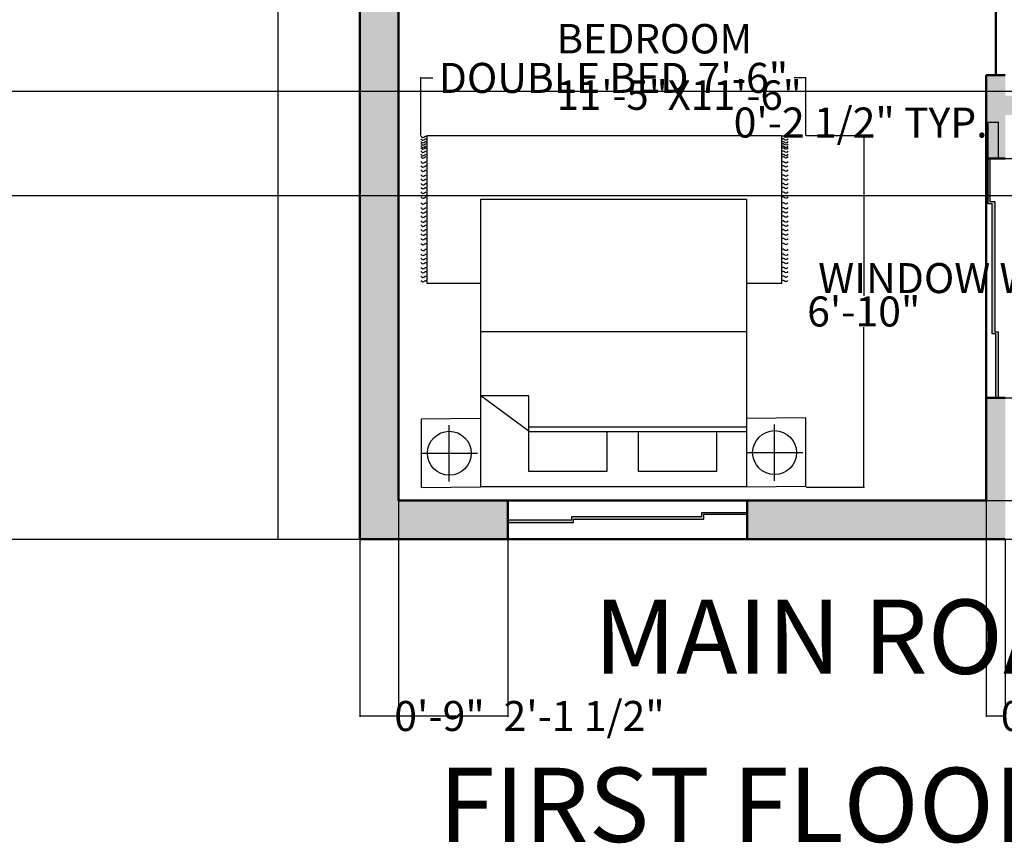
# Model space of a CAD drawing. Units: inches. Extents: x 48 to 822, y -191 to 651.
# Tile 2 of 13: x 429 to 659, y -191 to 1. Entities that reach past the tile are written whole.
import ezdxf

# ---------------------------------------------------------------- set-up
doc = ezdxf.new("R2010")
doc.units = ezdxf.units.IN
doc.header["$MEASUREMENT"] = 0
doc.layers.get('0').update_dxf_attribs({"color": 254})
for name, color, linetype, lineweight in [('A-ANNO-DIMS', 2, 'Continuous', 18), ('A-ANNO-TEXT', 3, 'Continuous', 25), ('A-AREA-IDEN', 7, 'Continuous', 25), ('A-FURN', 8, 'Continuous', 18), ('A-GLAZ', 4, 'Continuous', 25), ('A-WALL', 7, 'Continuous', 50), ('A-WALL-PATT', 8, 'Continuous', 13)]:
    doc.layers.add(name, color=color, linetype=linetype, lineweight=lineweight)
doc.layers.add('furniture', color=250, linetype='Continuous')
doc.styles.get("Standard").update_dxf_attribs({"font": 'arial.ttf'})
doc.dimstyles.get("Standard").update_dxf_attribs({"dimtxt": 7, "dimasz": 0.18, "dimexe": 0.18, "dimexo": 0.0625, "dimgap": 0.09, "dimtad": 0, "dimtih": 1, "dimtoh": 1, "dimzin": 0, "dimdsep": 46, "dimlunit": 3, "dimtxsty": 'Standard', "dimcen": 0.09, "dimadec": 0, "dimazin": 0, "dimtfac": 1, "dimtofl": 0, "dimtmove": 0, "dimatfit": 3, "dimfxl": 1, "dimtolj": 1, "dimtzin": 0, "dimarcsym": 0})

# ---------------------------------------------------------------- blocks, each defined once
blk = doc.blocks.new('CARPET')
at = {"layer": 'furniture'}
for p, q in [((-51.53, -98.11), (-51.53, -55.12)), ((-51.53, -55.12), (-41.27, -55.12)), ((36, -55.12), (51.55, -55.12)), ((51.55, -55.12), (51.55, -98.11)), ((51.55, -98.11), (-51.53, -98.11))]:
    blk.add_line(p, q, dxfattribs=at)
for points, knots in [([(-53.37, -55.99), (-53.22, -55.8), (-52.9, -55.41), (-52.34, -55.8), (-51.89, -56.08), (-51.65, -55.91), (-51.53, -55.83)], [0, 0, 0, 0, 0.653278, 1.290138, 1.740457, 2.114451, 2.114451, 2.114451, 2.114451]), ([(-53.37, -57.26), (-53.22, -57.07), (-52.9, -56.67), (-52.34, -57.07), (-51.89, -57.35), (-51.65, -57.17), (-51.53, -57.1)], [0, 0, 0, 0, 0.653278, 1.290138, 1.740457, 2.114451, 2.114451, 2.114451, 2.114451]), ([(53.37, -55.99), (53.22, -55.8), (52.9, -55.41), (52.34, -55.8), (51.89, -56.08), (51.65, -55.91), (51.53, -55.83)], [0, 0, 0, 0, 0.653278, 1.290138, 1.740457, 2.114451, 2.114451, 2.114451, 2.114451]), ([(53.37, -57.26), (53.22, -57.07), (52.9, -56.67), (52.34, -57.07), (51.89, -57.35), (51.65, -57.17), (51.53, -57.1)], [0, 0, 0, 0, 0.653278, 1.290138, 1.740457, 2.114451, 2.114451, 2.114451, 2.114451]), ([(-53.37, -58.59), (-53.22, -58.4), (-52.9, -58.01), (-52.34, -58.4), (-51.89, -58.68), (-51.65, -58.5), (-51.53, -58.43)], [0, 0, 0, 0, 0.653278, 1.290138, 1.740457, 2.114451, 2.114451, 2.114451, 2.114451]), ([(-53.37, -59.78), (-53.22, -59.58), (-52.9, -59.19), (-52.34, -59.58), (-51.89, -59.86), (-51.65, -59.69), (-51.53, -59.61)], [0, 0, 0, 0, 0.653278, 1.290138, 1.740457, 2.114451, 2.114451, 2.114451, 2.114451]), ([(53.37, -58.59), (53.22, -58.4), (52.9, -58.01), (52.34, -58.4), (51.89, -58.68), (51.65, -58.5), (51.53, -58.43)], [0, 0, 0, 0, 0.653278, 1.290138, 1.740457, 2.114451, 2.114451, 2.114451, 2.114451]), ([(53.37, -59.78), (53.22, -59.58), (52.9, -59.19), (52.34, -59.58), (51.89, -59.86), (51.65, -59.69), (51.53, -59.61)], [0, 0, 0, 0, 0.653278, 1.290138, 1.740457, 2.114451, 2.114451, 2.114451, 2.114451]), ([(-53.37, -61.22), (-53.22, -61.02), (-52.9, -60.63), (-52.34, -61.02), (-51.89, -61.3), (-51.65, -61.13), (-51.53, -61.05)], [0, 0, 0, 0, 0.653278, 1.290138, 1.740457, 2.114451, 2.114451, 2.114451, 2.114451]), ([(-53.37, -62.44), (-53.22, -62.25), (-52.9, -61.86), (-52.34, -62.25), (-51.89, -62.53), (-51.65, -62.36), (-51.53, -62.28)], [0, 0, 0, 0, 0.653278, 1.290138, 1.740457, 2.114451, 2.114451, 2.114451, 2.114451]), ([(53.37, -61.22), (53.22, -61.02), (52.9, -60.63), (52.34, -61.02), (51.89, -61.3), (51.65, -61.13), (51.53, -61.05)], [0, 0, 0, 0, 0.653278, 1.290138, 1.740457, 2.114451, 2.114451, 2.114451, 2.114451]), ([(53.37, -62.44), (53.22, -62.25), (52.9, -61.86), (52.34, -62.25), (51.89, -62.53), (51.65, -62.36), (51.53, -62.28)], [0, 0, 0, 0, 0.653278, 1.290138, 1.740457, 2.114451, 2.114451, 2.114451, 2.114451]), ([(-53.37, -63.63), (-53.22, -63.43), (-52.9, -63.04), (-52.34, -63.43), (-51.89, -63.72), (-51.65, -63.54), (-51.53, -63.46)], [0, 0, 0, 0, 0.653278, 1.290138, 1.740457, 2.114451, 2.114451, 2.114451, 2.114451]), ([(-53.37, -65.07), (-53.22, -64.87), (-52.9, -64.48), (-52.34, -64.87), (-51.89, -65.15), (-51.65, -64.98), (-51.53, -64.9)], [0, 0, 0, 0, 0.653278, 1.290138, 1.740457, 2.114451, 2.114451, 2.114451, 2.114451]), ([(53.37, -63.63), (53.22, -63.43), (52.9, -63.04), (52.34, -63.43), (51.89, -63.72), (51.65, -63.54), (51.53, -63.46)], [0, 0, 0, 0, 0.653278, 1.290138, 1.740457, 2.114451, 2.114451, 2.114451, 2.114451]), ([(53.37, -65.07), (53.22, -64.87), (52.9, -64.48), (52.34, -64.87), (51.89, -65.15), (51.65, -64.98), (51.53, -64.9)], [0, 0, 0, 0, 0.653278, 1.290138, 1.740457, 2.114451, 2.114451, 2.114451, 2.114451]), ([(-53.37, -66.76), (-53.22, -66.56), (-52.9, -66.17), (-52.34, -66.56), (-51.89, -66.84), (-51.65, -66.67), (-51.53, -66.59)], [0, 0, 0, 0, 0.653278, 1.290138, 1.740457, 2.114451, 2.114451, 2.114451, 2.114451]), ([(-53.37, -68.2), (-53.22, -68), (-52.9, -67.61), (-52.34, -68), (-51.89, -68.28), (-51.65, -68.11), (-51.53, -68.03)], [0, 0, 0, 0, 0.653278, 1.290138, 1.740457, 2.114451, 2.114451, 2.114451, 2.114451]), ([(53.37, -66.76), (53.22, -66.56), (52.9, -66.17), (52.34, -66.56), (51.89, -66.84), (51.65, -66.67), (51.53, -66.59)], [0, 0, 0, 0, 0.653278, 1.290138, 1.740457, 2.114451, 2.114451, 2.114451, 2.114451]), ([(53.37, -68.2), (53.22, -68), (52.9, -67.61), (52.34, -68), (51.89, -68.28), (51.65, -68.11), (51.53, -68.03)], [0, 0, 0, 0, 0.653278, 1.290138, 1.740457, 2.114451, 2.114451, 2.114451, 2.114451]), ([(-53.37, -69.53), (-53.22, -69.33), (-52.9, -68.94), (-52.34, -69.33), (-51.89, -69.61), (-51.65, -69.44), (-51.53, -69.36)], [0, 0, 0, 0, 0.653278, 1.290138, 1.740457, 2.114451, 2.114451, 2.114451, 2.114451]), ([(-53.37, -70.79), (-53.22, -70.6), (-52.9, -70.21), (-52.34, -70.6), (-51.89, -70.88), (-51.65, -70.7), (-51.53, -70.63)], [0, 0, 0, 0, 0.653278, 1.290138, 1.740457, 2.114451, 2.114451, 2.114451, 2.114451]), ([(53.37, -69.53), (53.22, -69.33), (52.9, -68.94), (52.34, -69.33), (51.89, -69.61), (51.65, -69.44), (51.53, -69.36)], [0, 0, 0, 0, 0.653278, 1.290138, 1.740457, 2.114451, 2.114451, 2.114451, 2.114451]), ([(53.37, -70.79), (53.22, -70.6), (52.9, -70.21), (52.34, -70.6), (51.89, -70.88), (51.65, -70.7), (51.53, -70.63)], [0, 0, 0, 0, 0.653278, 1.290138, 1.740457, 2.114451, 2.114451, 2.114451, 2.114451]), ([(-53.37, -72.12), (-53.22, -71.93), (-52.9, -71.54), (-52.34, -71.93), (-51.89, -72.21), (-51.65, -72.04), (-51.53, -71.96)], [0, 0, 0, 0, 0.653278, 1.290138, 1.740457, 2.114451, 2.114451, 2.114451, 2.114451]), ([(-53.37, -73.31), (-53.22, -73.11), (-52.9, -72.72), (-52.34, -73.11), (-51.89, -73.4), (-51.65, -73.22), (-51.53, -73.14)], [0, 0, 0, 0, 0.653278, 1.290138, 1.740457, 2.114451, 2.114451, 2.114451, 2.114451]), ([(-53.37, -74.75), (-53.22, -74.55), (-52.9, -74.16), (-52.34, -74.55), (-51.89, -74.83), (-51.65, -74.66), (-51.53, -74.58)], [0, 0, 0, 0, 0.653278, 1.290138, 1.740457, 2.114451, 2.114451, 2.114451, 2.114451]), ([(53.37, -72.12), (53.22, -71.93), (52.9, -71.54), (52.34, -71.93), (51.89, -72.21), (51.65, -72.04), (51.53, -71.96)], [0, 0, 0, 0, 0.653278, 1.290138, 1.740457, 2.114451, 2.114451, 2.114451, 2.114451]), ([(53.37, -73.31), (53.22, -73.11), (52.9, -72.72), (52.34, -73.11), (51.89, -73.4), (51.65, -73.22), (51.53, -73.14)], [0, 0, 0, 0, 0.653278, 1.290138, 1.740457, 2.114451, 2.114451, 2.114451, 2.114451]), ([(53.37, -74.75), (53.22, -74.55), (52.9, -74.16), (52.34, -74.55), (51.89, -74.83), (51.65, -74.66), (51.53, -74.58)], [0, 0, 0, 0, 0.653278, 1.290138, 1.740457, 2.114451, 2.114451, 2.114451, 2.114451]), ([(-53.37, -75.98), (-53.22, -75.78), (-52.9, -75.39), (-52.34, -75.78), (-51.89, -76.06), (-51.65, -75.89), (-51.53, -75.81)], [0, 0, 0, 0, 0.653278, 1.290138, 1.740457, 2.114451, 2.114451, 2.114451, 2.114451]), ([(-53.37, -77.16), (-53.22, -76.96), (-52.9, -76.57), (-52.34, -76.96), (-51.89, -77.25), (-51.65, -77.07), (-51.53, -76.99)], [0, 0, 0, 0, 0.653278, 1.290138, 1.740457, 2.114451, 2.114451, 2.114451, 2.114451]), ([(53.37, -75.98), (53.22, -75.78), (52.9, -75.39), (52.34, -75.78), (51.89, -76.06), (51.65, -75.89), (51.53, -75.81)], [0, 0, 0, 0, 0.653278, 1.290138, 1.740457, 2.114451, 2.114451, 2.114451, 2.114451]), ([(53.37, -77.16), (53.22, -76.96), (52.9, -76.57), (52.34, -76.96), (51.89, -77.25), (51.65, -77.07), (51.53, -76.99)], [0, 0, 0, 0, 0.653278, 1.290138, 1.740457, 2.114451, 2.114451, 2.114451, 2.114451]), ([(-53.37, -78.6), (-53.22, -78.4), (-52.9, -78.01), (-52.34, -78.4), (-51.89, -78.68), (-51.65, -78.51), (-51.53, -78.43)], [0, 0, 0, 0, 0.653278, 1.290138, 1.740457, 2.114451, 2.114451, 2.114451, 2.114451]), ([(-53.37, -80.29), (-53.22, -80.09), (-52.9, -79.7), (-52.34, -80.09), (-51.89, -80.37), (-51.65, -80.2), (-51.53, -80.12)], [0, 0, 0, 0, 0.653278, 1.290138, 1.740457, 2.114451, 2.114451, 2.114451, 2.114451]), ([(53.37, -78.6), (53.22, -78.4), (52.9, -78.01), (52.34, -78.4), (51.89, -78.68), (51.65, -78.51), (51.53, -78.43)], [0, 0, 0, 0, 0.653278, 1.290138, 1.740457, 2.114451, 2.114451, 2.114451, 2.114451]), ([(53.37, -80.29), (53.22, -80.09), (52.9, -79.7), (52.34, -80.09), (51.89, -80.37), (51.65, -80.2), (51.53, -80.12)], [0, 0, 0, 0, 0.653278, 1.290138, 1.740457, 2.114451, 2.114451, 2.114451, 2.114451]), ([(-53.37, -81.73), (-53.22, -81.53), (-52.9, -81.14), (-52.34, -81.53), (-51.89, -81.81), (-51.65, -81.64), (-51.53, -81.56)], [0, 0, 0, 0, 0.653278, 1.290138, 1.740457, 2.114451, 2.114451, 2.114451, 2.114451]), ([(-53.37, -83.06), (-53.22, -82.86), (-52.9, -82.47), (-52.34, -82.86), (-51.89, -83.14), (-51.65, -82.97), (-51.53, -82.89)], [0, 0, 0, 0, 0.653278, 1.290138, 1.740457, 2.114451, 2.114451, 2.114451, 2.114451]), ([(53.37, -81.73), (53.22, -81.53), (52.9, -81.14), (52.34, -81.53), (51.89, -81.81), (51.65, -81.64), (51.53, -81.56)], [0, 0, 0, 0, 0.653278, 1.290138, 1.740457, 2.114451, 2.114451, 2.114451, 2.114451]), ([(53.37, -83.06), (53.22, -82.86), (52.9, -82.47), (52.34, -82.86), (51.89, -83.14), (51.65, -82.97), (51.53, -82.89)], [0, 0, 0, 0, 0.653278, 1.290138, 1.740457, 2.114451, 2.114451, 2.114451, 2.114451]), ([(-53.37, -84.18), (-53.22, -83.99), (-52.9, -83.6), (-52.34, -83.99), (-51.89, -84.27), (-51.65, -84.09), (-51.53, -84.02)], [0, 0, 0, 0, 0.653278, 1.290138, 1.740457, 2.114451, 2.114451, 2.114451, 2.114451]), ([(-53.37, -85.51), (-53.22, -85.32), (-52.9, -84.93), (-52.34, -85.32), (-51.89, -85.6), (-51.65, -85.42), (-51.53, -85.35)], [0, 0, 0, 0, 0.653278, 1.290138, 1.740457, 2.114451, 2.114451, 2.114451, 2.114451]), ([(53.37, -84.18), (53.22, -83.99), (52.9, -83.6), (52.34, -83.99), (51.89, -84.27), (51.65, -84.09), (51.53, -84.02)], [0, 0, 0, 0, 0.653278, 1.290138, 1.740457, 2.114451, 2.114451, 2.114451, 2.114451]), ([(53.37, -85.51), (53.22, -85.32), (52.9, -84.93), (52.34, -85.32), (51.89, -85.6), (51.65, -85.42), (51.53, -85.35)], [0, 0, 0, 0, 0.653278, 1.290138, 1.740457, 2.114451, 2.114451, 2.114451, 2.114451]), ([(-53.37, -86.7), (-53.22, -86.5), (-52.9, -86.11), (-52.34, -86.5), (-51.89, -86.78), (-51.65, -86.61), (-51.53, -86.53)], [0, 0, 0, 0, 0.653278, 1.290138, 1.740457, 2.114451, 2.114451, 2.114451, 2.114451]), ([(-53.37, -88.14), (-53.22, -87.94), (-52.9, -87.55), (-52.34, -87.94), (-51.89, -88.22), (-51.65, -88.05), (-51.53, -87.97)], [0, 0, 0, 0, 0.653278, 1.290138, 1.740457, 2.114451, 2.114451, 2.114451, 2.114451]), ([(53.37, -86.7), (53.22, -86.5), (52.9, -86.11), (52.34, -86.5), (51.89, -86.78), (51.65, -86.61), (51.53, -86.53)], [0, 0, 0, 0, 0.653278, 1.290138, 1.740457, 2.114451, 2.114451, 2.114451, 2.114451]), ([(53.37, -88.14), (53.22, -87.94), (52.9, -87.55), (52.34, -87.94), (51.89, -88.22), (51.65, -88.05), (51.53, -87.97)], [0, 0, 0, 0, 0.653278, 1.290138, 1.740457, 2.114451, 2.114451, 2.114451, 2.114451]), ([(-53.37, -89.36), (-53.22, -89.17), (-52.9, -88.78), (-52.34, -89.17), (-51.89, -89.45), (-51.65, -89.28), (-51.53, -89.2)], [0, 0, 0, 0, 0.653278, 1.290138, 1.740457, 2.114451, 2.114451, 2.114451, 2.114451]), ([(-53.37, -90.55), (-53.22, -90.35), (-52.9, -89.96), (-52.34, -90.35), (-51.89, -90.64), (-51.65, -90.46), (-51.53, -90.38)], [0, 0, 0, 0, 0.653278, 1.290138, 1.740457, 2.114451, 2.114451, 2.114451, 2.114451]), ([(-53.37, -91.99), (-53.22, -91.79), (-52.9, -91.4), (-52.34, -91.79), (-51.89, -92.07), (-51.65, -91.9), (-51.53, -91.82)], [0, 0, 0, 0, 0.653278, 1.290138, 1.740457, 2.114451, 2.114451, 2.114451, 2.114451]), ([(53.37, -89.36), (53.22, -89.17), (52.9, -88.78), (52.34, -89.17), (51.89, -89.45), (51.65, -89.28), (51.53, -89.2)], [0, 0, 0, 0, 0.653278, 1.290138, 1.740457, 2.114451, 2.114451, 2.114451, 2.114451]), ([(53.37, -90.55), (53.22, -90.35), (52.9, -89.96), (52.34, -90.35), (51.9, -90.63), (51.66, -90.47), (51.55, -90.4)], [0, 0, 0, 0, 0.653278, 1.290138, 1.740457, 2.0926, 2.0926, 2.0926, 2.0926]), ([(53.37, -91.99), (53.22, -91.79), (52.9, -91.4), (52.34, -91.79), (51.9, -92.07), (51.66, -91.91), (51.55, -91.83)], [0, 0, 0, 0, 0.653278, 1.290138, 1.740457, 2.0926, 2.0926, 2.0926, 2.0926]), ([(-53.37, -92.69), (-53.22, -92.48), (-52.9, -92.08), (-52.35, -92.49), (-51.89, -92.77), (-51.65, -92.6), (-51.53, -92.52)], [0, 0, 0, 0, 0.663904, 1.307406, 1.757725, 2.131719, 2.131719, 2.131719, 2.131719]), ([(-53.37, -93.61), (-53.22, -93.42), (-52.9, -93.03), (-52.34, -93.42), (-51.89, -93.7), (-51.65, -93.52), (-51.53, -93.45)], [0, 0, 0, 0, 0.653278, 1.290138, 1.740457, 2.114451, 2.114451, 2.114451, 2.114451]), ([(-53.37, -94.55), (-53.22, -94.35), (-52.9, -93.96), (-52.34, -94.35), (-51.89, -94.63), (-51.65, -94.46), (-51.53, -94.38)], [0, 0, 0, 0, 0.653278, 1.290138, 1.740457, 2.114451, 2.114451, 2.114451, 2.114451]), ([(53.37, -92.69), (53.22, -92.49), (52.9, -92.09), (52.34, -92.49), (51.9, -92.77), (51.66, -92.61), (51.55, -92.53)], [0, 0, 0, 0, 0.656792, 1.295826, 1.746145, 2.098292, 2.098292, 2.098292, 2.098292]), ([(53.37, -93.66), (53.22, -93.46), (52.9, -93.07), (52.34, -93.46), (51.9, -93.74), (51.66, -93.58), (51.55, -93.5)], [0, 0, 0, 0, 0.653278, 1.290138, 1.740457, 2.0926, 2.0926, 2.0926, 2.0926]), ([(53.37, -94.59), (53.22, -94.4), (52.9, -94.01), (52.34, -94.4), (51.9, -94.68), (51.66, -94.51), (51.55, -94.44)], [0, 0, 0, 0, 0.653278, 1.290138, 1.740457, 2.0926, 2.0926, 2.0926, 2.0926]), ([(-53.37, -95.05), (-53.22, -94.85), (-52.9, -94.46), (-52.34, -94.85), (-51.89, -95.14), (-51.65, -94.96), (-51.53, -94.88)], [0, 0, 0, 0, 0.653278, 1.290138, 1.740457, 2.114451, 2.114451, 2.114451, 2.114451]), ([(-53.37, -95.73), (-53.22, -95.54), (-52.9, -95.15), (-52.34, -95.54), (-51.89, -95.82), (-51.65, -95.65), (-51.53, -95.57)], [0, 0, 0, 0, 0.653278, 1.290138, 1.740457, 2.114451, 2.114451, 2.114451, 2.114451]), ([(-53.37, -96.38), (-53.22, -96.18), (-52.9, -95.79), (-52.34, -96.18), (-51.89, -96.47), (-51.65, -96.29), (-51.53, -96.21)], [0, 0, 0, 0, 0.653278, 1.290138, 1.740457, 2.114451, 2.114451, 2.114451, 2.114451]), ([(-53.37, -97.17), (-53.22, -96.98), (-52.9, -96.59), (-52.34, -96.98), (-51.89, -97.26), (-51.65, -97.08), (-51.53, -97.01)], [0, 0, 0, 0, 0.653278, 1.290138, 1.740457, 2.114451, 2.114451, 2.114451, 2.114451]), ([(53.37, -95.78), (53.22, -95.58), (52.9, -95.19), (52.34, -95.58), (51.89, -95.86), (51.65, -95.69), (51.53, -95.61)], [0, 0, 0, 0, 0.653278, 1.290138, 1.740457, 2.114451, 2.114451, 2.114451, 2.114451]), ([(53.37, -96.43), (53.22, -96.23), (52.9, -95.84), (52.34, -96.23), (51.89, -96.51), (51.65, -96.34), (51.53, -96.26)], [0, 0, 0, 0, 0.653278, 1.290138, 1.740457, 2.114451, 2.114451, 2.114451, 2.114451]), ([(53.37, -97.22), (53.22, -97.02), (52.9, -96.63), (52.34, -97.02), (51.89, -97.3), (51.65, -97.13), (51.53, -97.05)], [0, 0, 0, 0, 0.653278, 1.290138, 1.740457, 2.114451, 2.114451, 2.114451, 2.114451]), ([(53.37, -95.1), (53.22, -94.9), (52.9, -94.51), (52.34, -94.9), (51.9, -95.18), (51.66, -95.02), (51.55, -94.94)], [0, 0, 0, 0, 0.653278, 1.290138, 1.740457, 2.0926, 2.0926, 2.0926, 2.0926]), ([(-53.37, -97.99), (-53.22, -97.79), (-52.9, -97.4), (-52.34, -97.79), (-51.89, -98.08), (-51.65, -97.9), (-51.53, -97.82)], [0, 0, 0, 0, 0.653278, 1.290138, 1.740457, 2.114451, 2.114451, 2.114451, 2.114451]), ([(53.37, -97.99), (53.22, -97.79), (52.9, -97.4), (52.34, -97.79), (51.89, -98.08), (51.65, -97.9), (51.53, -97.82)], [0, 0, 0, 0, 0.653278, 1.290138, 1.740457, 2.114451, 2.114451, 2.114451, 2.114451])]:
    blk.add_open_spline(points, degree=3, knots=knots, dxfattribs=at)
blk = doc.blocks.new('A$C58D270C6')
at = {"layer": 'furniture'}
for p, q in [((9.09, 124.13), (9.09, 108.87)), ((1.46, 116.5), (16.73, 116.5)), ((14.97, 94.84), (24.62, 107.92)), ((24.62, 94.93), (24.62, 107.92)), ((42.08, 108), (42.08, 36)), ((14.97, 94.93), (24.62, 94.93)), ((14.97, 94.84), (14.97, 36)), ((16.22, 94.93), (16.22, 36)), ((9.25, 36), (9.25, 20.74)), ((1.62, 28.37), (16.88, 28.37))]:
    blk.add_line(p, q, dxfattribs=at)
for points in [[(18.5, 108), (18.34, 124.13), (-0.16, 124.13), (0, 108)], [(0, 108), (77.91, 108), (77.91, 36), (0, 36)], [(4.09, 94.93), (14.97, 94.93), (14.97, 73.83), (4.09, 73.83)], [(4.09, 65.23), (14.97, 65.23), (14.97, 44.13), (4.09, 44.13)], [(18.65, 19.87), (18.5, 36), (0, 36), (0.16, 19.87)]]:
    blk.add_lwpolyline(points, close=True, dxfattribs=at)
for centre in [(9.09, 116.5), (9.25, 28.37)]:
    blk.add_circle(centre, 5.95, dxfattribs=at)
at = {"layer": 'furniture', "xscale": 0.9312884925094044, "yscale": 0.9312884925094044, "zscale": 0.9312884925094044, "rotation": 90}
blk.add_blockref('CARPET', (3.79, 74.47), dxfattribs=at)
blk = doc.blocks.new('*D19')
at = {"layer": 'A-ANNO-DIMS', "color": 0, "lineweight": -2, "transparency": 16777216}
for p, q in [((489.56, 599.69), (489.41, 599.69)), ((489.59, 599.51), (489.59, 243.35)), ((489.59, -120.13), (489.59, 236.02)), ((489.56, -120.31), (489.41, -120.31))]:
    blk.add_line(p, q, dxfattribs=at)
at = {"layer": 'A-ANNO-DIMS', "color": 0, "transparency": 16777216}
for points in [[(489.56, 599.51), (489.62, 599.51), (489.59, 599.69)], [(489.56, -120.13), (489.62, -120.13), (489.59, -120.31)]]:
    blk.add_solid(points, dxfattribs=at)
at = {"layer": 'Defpoints', "color": 0, "transparency": 16777216}
for p in [(489.62, 599.69), (489.59, -120.31), (489.62, -120.31)]:
    blk.add_point(p, dxfattribs=at)
at = {"layer": 'A-ANNO-DIMS', "color": 0, "transparency": 16777216, "insert": (489.59, 239.69), "char_height": 7, "attachment_point": 5}
blk.add_mtext("\\A1;60'", dxfattribs=at)
blk = doc.blocks.new('WIN-1500')
for p, q in [((300.62, 546.44), (315.51, 546.44)), ((315.51, 546.44), (315.51, 547.24)), ((315.51, 547.24), (345.84, 547.24)), ((315.95, 545.8), (315.95, 546.59)), ((315.95, 546.59), (346.31, 546.59)), ((345.84, 547.24), (345.84, 548.17)), ((345.84, 548.17), (356.45, 548.17)), ((346.31, 546.59), (346.31, 547.73)), ((346.31, 547.73), (356.45, 547.73)), ((300.62, 545.8), (315.95, 545.8))]:
    blk.add_line(p, q)
blk = doc.blocks.new('*D28')
at = {"layer": 'A-ANNO-DIMS', "color": 0, "lineweight": -2, "transparency": 16777216}
for p, q in [((657.56, -31.5), (666.06, -31.5)), ((665.88, -31.68), (665.88, -55.7)), ((665.88, -87.15), (665.88, -63.13)), ((657.56, -87.33), (666.06, -87.33))]:
    blk.add_line(p, q, dxfattribs=at)
at = {"layer": 'A-ANNO-DIMS', "color": 0, "transparency": 16777216}
for points in [[(665.85, -31.68), (665.91, -31.68), (665.88, -31.5)], [(665.85, -87.15), (665.91, -87.15), (665.88, -87.33)]]:
    blk.add_solid(points, dxfattribs=at)
at = {"layer": 'Defpoints', "color": 0, "transparency": 16777216}
for p in [(657.5, -31.5), (665.88, -31.5), (657.5, -87.33)]:
    blk.add_point(p, dxfattribs=at)
at = {"layer": 'A-ANNO-DIMS', "color": 0, "transparency": 16777216, "insert": (665.88, -59.42), "char_height": 7, "attachment_point": 5}
blk.add_mtext('\\A1;WINDOW W1 4\'-8" TYP.', dxfattribs=at)
blk = doc.blocks.new('*D29')
at = {"layer": 'A-ANNO-DIMS', "color": 0, "lineweight": -2, "transparency": 16777216}
for p, q in [((655.13, -31.44), (655.13, -22.95)), ((657.5, -31.44), (657.5, -22.95)), ((655.13, -23.13), (654.95, -23.13)), ((657.32, -23.13), (655.31, -23.13))]:
    blk.add_line(p, q, dxfattribs=at)
at = {"layer": 'A-ANNO-DIMS', "color": 0, "transparency": 16777216}
for points in [[(655.31, -23.1), (655.31, -23.16), (655.13, -23.13)], [(657.32, -23.1), (657.32, -23.16), (657.5, -23.13)]]:
    blk.add_solid(points, dxfattribs=at)
at = {"layer": 'Defpoints', "color": 0, "transparency": 16777216}
for p in [(655.13, -23.13), (655.13, -31.5), (657.5, -31.5)]:
    blk.add_point(p, dxfattribs=at)
at = {"layer": 'A-ANNO-DIMS', "color": 0, "transparency": 16777216, "insert": (625.37, -23.13), "char_height": 7, "attachment_point": 5}
blk.add_mtext('\\A1;0\'-2 1/2" TYP.', dxfattribs=at)
blk = doc.blocks.new('*D42')
at = {"layer": 'A-ANNO-DIMS', "color": 0, "lineweight": -2, "transparency": 16777216}
for p, q in [((522.85, -26.13), (522.85, -12.54)), ((523.03, -12.72), (525.64, -12.72)), ((612.45, -12.72), (609.84, -12.72)), ((612.63, -26.13), (612.63, -12.54))]:
    blk.add_line(p, q, dxfattribs=at)
at = {"layer": 'A-ANNO-DIMS', "color": 0, "transparency": 16777216}
for points in [[(523.03, -12.69), (523.03, -12.75), (522.85, -12.72)], [(612.45, -12.69), (612.45, -12.75), (612.63, -12.72)]]:
    blk.add_solid(points, dxfattribs=at)
at = {"layer": 'Defpoints', "color": 0, "transparency": 16777216}
for p in [(522.85, -12.72), (522.85, -26.19), (612.63, -26.19)]:
    blk.add_point(p, dxfattribs=at)
at = {"layer": 'A-ANNO-DIMS', "color": 0, "transparency": 16777216, "insert": (567.74, -12.72), "char_height": 7, "attachment_point": 5}
blk.add_mtext('\\A1;DOUBLE BED 7\'-6"', dxfattribs=at)
blk = doc.blocks.new('*D43')
at = {"layer": 'A-ANNO-DIMS', "color": 0, "lineweight": -2, "transparency": 16777216}
for p, q in [((612.69, -26.19), (626.28, -26.19)), ((626.1, -26.37), (626.1, -63.54)), ((626.1, -108.04), (626.1, -70.87)), ((612.69, -108.22), (626.28, -108.22))]:
    blk.add_line(p, q, dxfattribs=at)
at = {"layer": 'A-ANNO-DIMS', "color": 0, "transparency": 16777216}
for points in [[(626.07, -26.37), (626.13, -26.37), (626.1, -26.19)], [(626.07, -108.04), (626.13, -108.04), (626.1, -108.22)]]:
    blk.add_solid(points, dxfattribs=at)
at = {"layer": 'Defpoints', "color": 0, "transparency": 16777216}
for p in [(612.63, -26.19), (626.1, -26.19), (612.63, -108.22)]:
    blk.add_point(p, dxfattribs=at)
at = {"layer": 'A-ANNO-DIMS', "color": 0, "transparency": 16777216, "insert": (626.1, -67.21), "char_height": 7, "attachment_point": 5}
blk.add_mtext('\\A1;6\'-10"', dxfattribs=at)
blk = doc.blocks.new('*D87')
at = {"layer": 'A-ANNO-DIMS', "color": 0, "lineweight": -2, "transparency": 16777216}
for p, q in [((361.01, 6.84), (790.04, 6.84)), ((789.86, 6.66), (789.86, -0.78)), ((789.86, -15.63), (789.86, -8.2)), ((361.01, -15.81), (790.04, -15.81))]:
    blk.add_line(p, q, dxfattribs=at)
at = {"layer": 'A-ANNO-DIMS', "color": 0, "transparency": 16777216}
for points in [[(789.83, 6.66), (789.89, 6.66), (789.86, 6.84)], [(789.83, -15.63), (789.89, -15.63), (789.86, -15.81)]]:
    blk.add_solid(points, dxfattribs=at)
at = {"layer": 'Defpoints', "color": 0, "transparency": 16777216}
for p in [(360.95, 6.84), (360.95, -15.81), (789.86, -15.81)]:
    blk.add_point(p, dxfattribs=at)
at = {"layer": 'A-ANNO-DIMS', "color": 0, "transparency": 16777216, "insert": (789.86, -4.49), "char_height": 7, "attachment_point": 5}
blk.add_mtext('\\A1;1\'-10 1/2"', dxfattribs=at)
blk = doc.blocks.new('*D88')
at = {"layer": 'A-ANNO-DIMS', "color": 0, "lineweight": -2, "transparency": 16777216}
for p, q in [((361.01, -15.81), (790.04, -15.81)), ((789.86, -15.99), (789.86, -64.35)), ((789.86, -120.13), (789.86, -71.77)), ((365.51, -120.31), (790.04, -120.31))]:
    blk.add_line(p, q, dxfattribs=at)
at = {"layer": 'A-ANNO-DIMS', "color": 0, "transparency": 16777216}
for points in [[(789.83, -15.99), (789.89, -15.99), (789.86, -15.81)], [(789.83, -120.13), (789.89, -120.13), (789.86, -120.31)]]:
    blk.add_solid(points, dxfattribs=at)
at = {"layer": 'Defpoints', "color": 0, "transparency": 16777216}
for p in [(360.95, -15.81), (365.45, -120.31), (789.86, -120.31)]:
    blk.add_point(p, dxfattribs=at)
at = {"layer": 'A-ANNO-DIMS', "color": 0, "transparency": 16777216, "insert": (789.86, -68.06), "char_height": 7, "attachment_point": 5}
blk.add_mtext('\\A1;8\'-8 1/2"', dxfattribs=at)
blk = doc.blocks.new('*D93')
at = {"layer": 'A-ANNO-DIMS', "color": 0, "lineweight": -2, "transparency": 16777216}
for p, q in [((271.51, 15.7), (790.04, 15.7)), ((789.86, 15.52), (789.86, -8.55)), ((789.86, -39.95), (789.86, -15.88)), ((271.51, -40.13), (790.04, -40.13))]:
    blk.add_line(p, q, dxfattribs=at)
at = {"layer": 'A-ANNO-DIMS', "color": 0, "transparency": 16777216}
for points in [[(789.83, 15.52), (789.89, 15.52), (789.86, 15.7)], [(789.83, -39.95), (789.89, -39.95), (789.86, -40.13)]]:
    blk.add_solid(points, dxfattribs=at)
at = {"layer": 'Defpoints', "color": 0, "transparency": 16777216}
for p in [(271.45, 15.7), (271.45, -40.13), (789.86, -40.13)]:
    blk.add_point(p, dxfattribs=at)
at = {"layer": 'A-ANNO-DIMS', "color": 0, "transparency": 16777216, "insert": (789.86, -12.22), "char_height": 7, "attachment_point": 5}
blk.add_mtext('\\A1;4\'-8"', dxfattribs=at)
blk = doc.blocks.new('*D101')
at = {"layer": 'A-ANNO-DIMS', "color": 0, "lineweight": -2, "transparency": 16777216}
for p, q in [((517.61, -111.38), (517.61, -161.74)), ((508.61, -120.38), (508.61, -161.74)), ((508.79, -161.56), (517.43, -161.56)), ((517.61, -161.56), (517.79, -161.56))]:
    blk.add_line(p, q, dxfattribs=at)
at = {"layer": 'A-ANNO-DIMS', "color": 0, "transparency": 16777216}
for points in [[(508.79, -161.53), (508.79, -161.59), (508.61, -161.56)], [(517.43, -161.53), (517.43, -161.59), (517.61, -161.56)]]:
    blk.add_solid(points, dxfattribs=at)
at = {"layer": 'Defpoints', "color": 0, "transparency": 16777216}
for p in [(517.61, -111.31), (508.61, -120.31), (517.61, -161.56)]:
    blk.add_point(p, dxfattribs=at)
at = {"layer": 'A-ANNO-DIMS', "color": 0, "transparency": 16777216, "insert": (527.18, -161.56), "char_height": 7, "attachment_point": 5}
blk.add_mtext('\\A1;0\'-9"', dxfattribs=at)
blk = doc.blocks.new('*D102')
at = {"layer": 'A-ANNO-DIMS', "color": 0, "lineweight": -2, "transparency": 16777216}
for p, q in [((654.61, -111.38), (654.61, -161.74)), ((659.11, -120.38), (659.11, -161.74)), ((654.79, -161.56), (658.93, -161.56)), ((659.11, -161.56), (659.29, -161.56))]:
    blk.add_line(p, q, dxfattribs=at)
at = {"layer": 'A-ANNO-DIMS', "color": 0, "transparency": 16777216}
for points in [[(654.79, -161.53), (654.79, -161.59), (654.61, -161.56)], [(658.93, -161.53), (658.93, -161.59), (659.11, -161.56)]]:
    blk.add_solid(points, dxfattribs=at)
at = {"layer": 'Defpoints', "color": 0, "transparency": 16777216}
for p in [(654.61, -111.31), (659.11, -120.31), (659.11, -161.56)]:
    blk.add_point(p, dxfattribs=at)
at = {"layer": 'A-ANNO-DIMS', "color": 0, "transparency": 16777216, "insert": (676.84, -161.56), "char_height": 7, "attachment_point": 5}
blk.add_mtext('\\A1;0\'-4 1/2"', dxfattribs=at)
blk = doc.blocks.new('*D103')
at = {"layer": 'A-ANNO-DIMS', "color": 0, "lineweight": -2, "transparency": 16777216}
for p, q in [((517.61, -111.38), (517.61, -161.74)), ((543.11, -111.38), (543.11, -161.74)), ((517.79, -161.56), (542.93, -161.56)), ((543.11, -161.56), (543.29, -161.56))]:
    blk.add_line(p, q, dxfattribs=at)
at = {"layer": 'A-ANNO-DIMS', "color": 0, "transparency": 16777216}
for points in [[(517.79, -161.53), (517.79, -161.59), (517.61, -161.56)], [(542.93, -161.53), (542.93, -161.59), (543.11, -161.56)]]:
    blk.add_solid(points, dxfattribs=at)
at = {"layer": 'Defpoints', "color": 0, "transparency": 16777216}
for p in [(517.61, -111.31), (543.11, -111.31), (543.11, -161.56)]:
    blk.add_point(p, dxfattribs=at)
at = {"layer": 'A-ANNO-DIMS', "color": 0, "transparency": 16777216, "insert": (560.9, -161.56), "char_height": 7, "attachment_point": 5}
blk.add_mtext('\\A1;2\'-1 1/2"', dxfattribs=at)
blk = doc.blocks.new('*D117')
at = {"layer": 'A-ANNO-DIMS', "color": 0, "lineweight": -2, "transparency": 16777216}
for p, q in [((517.67, 38.69), (790.04, 38.69)), ((789.86, 38.51), (789.86, -32.65)), ((789.86, -111.13), (789.86, -39.98)), ((517.67, -111.31), (790.04, -111.31))]:
    blk.add_line(p, q, dxfattribs=at)
at = {"layer": 'A-ANNO-DIMS', "color": 0, "transparency": 16777216}
for points in [[(789.83, 38.51), (789.89, 38.51), (789.86, 38.69)], [(789.83, -111.13), (789.89, -111.13), (789.86, -111.31)]]:
    blk.add_solid(points, dxfattribs=at)
at = {"layer": 'Defpoints', "color": 0, "transparency": 16777216}
for p in [(517.61, 38.69), (517.61, -111.31), (789.86, -111.31)]:
    blk.add_point(p, dxfattribs=at)
at = {"layer": 'A-ANNO-DIMS', "color": 0, "transparency": 16777216, "insert": (789.86, -36.31), "char_height": 7, "attachment_point": 5}
blk.add_mtext('\\A1;12\'-6"', dxfattribs=at)

msp = doc.modelspace()

# ---------------------------------------------------------------- hatches: boundary and pattern name
at = {"layer": 'A-WALL-PATT'}
h = msp.add_hatch(color=256, dxfattribs=at)
h.dxf.hatch_style = 1
h.paths.add_polyline_path([(614.11, 432.437), (609.61, 432.437), (609.61, 376.187), (535.284, 376.187), (535.284, 371.687), (547.61, 371.687), (547.61, 359.12), (552.11, 359.12), (552.11, 371.687), (609.61, 371.687), (609.61, 335.687), (614.11, 335.687)], flags=17)
h.paths.add_polyline_path([(614.11, 434.687), (609.61, 434.687), (609.61, 432.437), (614.11, 432.437)], flags=17)
h.paths.add_polyline_path([(573.934, 434.687), (517.61, 434.687), (517.61, 590.687), (650.61, 590.687), (650.61, 585.522), (655.11, 585.522), (655.11, 590.687), (739.61, 590.687), (739.61, 548.687), (655.11, 548.687), (655.11, 550.72), (650.61, 550.72), (650.61, 458.608), (655.11, 458.608), (655.11, 544.187), (739.61, 544.187), (739.61, 434.541), (650.61, 434.541), (650.61, 430.041), (739.61, 430.041), (739.61, -16.844), (729.973, -16.844), (729.973, -21.344), (748.61, -21.344), (748.61, 599.687), (508.61, 599.687), (508.61, -120.313), (543.114, -120.313), (543.114, -111.313), (517.61, -111.313), (517.61, 38.687), (607.29, 38.687), (607.29, 43.187), (517.61, 43.187), (517.61, 97.187), (654.61, 97.187), (654.61, 30.562), (659.11, 30.562), (659.11, 101.895), (654.61, 101.895), (654.61, 101.687), (517.61, 101.687), (517.61, 221.687), (654.61, 221.687), (654.61, 218.066), (659.11, 218.066), (659.11, 226.187), (517.61, 226.187), (517.61, 295.187), (614.11, 295.187), (648.087, 295.187), (661.07, 295.187), (661.07, 299.687), (614.11, 299.687), (552.11, 299.687), (552.11, 341.37), (547.61, 341.37), (547.61, 299.687), (517.61, 299.687), (517.61, 371.687), (517.534, 371.687), (517.534, 376.187), (517.61, 430.187), (573.934, 430.187)])
h.paths.add_polyline_path([(659.11, -87.328), (654.61, -87.328), (654.61, -111.313), (598.94, -111.313), (598.94, -120.313), (659.11, -120.313)], flags=0)
h.paths.add_polyline_path([(671.266, -16.844), (659.11, -16.844), (659.11, -12.05), (654.61, -12.05), (654.61, -31.502), (659.11, -31.502), (659.11, -21.344), (671.266, -21.344)], flags=17)
h.paths.add_polyline_path([(606.11, 97.187), (601.61, 97.187), (601.61, 75.902), (606.11, 75.902)], flags=17)
h.paths.add_polyline_path([(659.11, 169.875), (654.61, 169.875), (654.61, 157.721), (659.11, 157.721)], flags=17)
h = msp.add_hatch(color=256, dxfattribs=at)
h.dxf.hatch_style = 1
h.paths.add_polyline_path([(216.887, -62.023), (227.03, -62.023), (227.03, -61.583), (216.418, -61.583), (216.418, -62.508), (186.092, -62.508), (186.092, -63.313), (171.204, -63.313), (171.204, -63.954), (186.533, -63.954), (186.533, -63.161), (216.887, -63.161)])
h.paths.add_polyline_path([(588.796, -114.523), (598.94, -114.523), (598.94, -114.083), (588.328, -114.083), (588.328, -115.008), (558.002, -115.008), (558.002, -115.813), (543.114, -115.813), (543.114, -116.454), (558.443, -116.454), (558.443, -115.661), (588.796, -115.661)])
h.paths.add_polyline_path([(656.709, -41.646), (655.571, -41.646), (655.571, -31.502), (655.131, -31.502), (655.131, -42.114), (656.055, -42.114), (656.055, -72.44), (656.86, -72.44), (656.86, -87.328), (657.501, -87.328), (657.501, -72), (656.709, -72)])
h.paths.add_polyline_path([(273.549, 5.552), (272.411, 5.552), (272.411, 15.696), (271.971, 15.696), (271.971, 5.084), (272.896, 5.084), (272.896, -25.242), (273.701, -25.242), (273.701, -40.13), (274.342, -40.13), (274.342, -24.802), (273.549, -24.802)])
h = msp.add_hatch(color=256, dxfattribs=at)
h.dxf.hatch_style = 1
h.paths.add_polyline_path([(659.11, -87.328), (654.61, -87.328), (654.61, -111.313), (598.94, -111.313), (598.94, -120.313), (659.11, -120.313)])

# ---------------------------------------------------------------- linework, layer by layer
at = {"layer": 'A-WALL'}
for p, q in [((508.61, -120.313), (508.61, 599.687)), ((517.61, -111.313), (517.61, 38.687)), ((656.86, 30.562), (656.86, -12.05)), ((654.61, -111.313), (654.61, -12.05)), ((654.61, -12.05), (659.11, -12.05)), ((659.11, -31.502), (654.61, -31.502)), ((654.61, -31.502), (654.61, -87.328)), ((654.61, -87.328), (659.11, -87.328)), ((654.61, -111.313), (517.61, -111.313)), ((543.114, -111.313), (543.114, -120.313)), ((598.94, -111.313), (543.114, -111.313)), ((598.94, -120.313), (598.94, -111.313)), ((659.11, -120.313), (508.61, -120.313)), ((543.114, -120.313), (598.94, -120.313))]:
    msp.add_line(p, q, dxfattribs=at)

# ---------------------------------------------------------------- block references
at = {"layer": 'A-FURN', "xscale": 0.8606489328555001, "yscale": 0.8606489328555001, "zscale": 0.8606489328555001, "rotation": 90}
msp.add_blockref('A$C58D270C6', (629.73, -108.089), dxfattribs=at)
at = {"layer": 'A-GLAZ', "rotation": 90}
msp.add_blockref('WIN-1500', (1203.297, -387.953), dxfattribs=at)
at = {"layer": 'A-GLAZ'}
msp.add_blockref('WIN-1500', (242.489, -662.249), dxfattribs=at)

# ---------------------------------------------------------------- texts
at = {"layer": 'A-ANNO-TEXT'}
for s, height, p in [('MAIN ROAD', 17.3215, (563.17, -151.725)), ('FIRST FLOOR PLAN', 17.32149, (527.002, -190.95))]:
    msp.add_text(s, height=height, dxfattribs=at).set_placement(p)
at = {"layer": 'A-AREA-IDEN'}
for s, height, p in [('BEDROOM', 6.866, (554.506, -7.019)), ('11\'-5"X11\'-6"', 6.86603, (554.506, -20.178))]:
    msp.add_text(s, height=height, dxfattribs=at).set_placement(p)

# ---------------------------------------------------------------- dimensions: what is measured, and where the dimension line sits
at = {"layer": 'A-ANNO-DIMS'}
for base, p1, p2, override, picture, middle in [((489.59, -120.313), (489.619, 599.687), (489.619, -120.313), {"dimclrd": 0, "dimclre": 0, "dimclrt": 0}, '*D19', (489.59, 239.687)), ((789.86, -111.313), (517.61, 38.687), (517.61, -111.313), {"dimdec": 1, "dimlfac": 1, "dimrnd": 0, "dimzin": 1, "dimdsep": 46, "dimlunit": 4, "dimfrac": 2}, '*D117', (789.86, -36.313)), ((789.86, -40.13), (271.451, 15.696), (271.451, -40.13), {"dimdec": 1, "dimlfac": 1, "dimrnd": 0, "dimzin": 1, "dimdsep": 46, "dimlunit": 4, "dimfrac": 2}, '*D93', (789.86, -12.217)), ((789.86, -15.813), (360.951, 6.835), (360.951, -15.813), {"dimdec": 1, "dimlfac": 1, "dimrnd": 0, "dimzin": 1, "dimdsep": 46, "dimlunit": 4, "dimfrac": 2}, '*D87', (789.86, -4.489)), ((789.86, -120.313), (360.951, -15.813), (365.451, -120.313), {"dimdec": 1, "dimlfac": 1, "dimrnd": 0, "dimzin": 1, "dimdsep": 46, "dimlunit": 4, "dimfrac": 2}, '*D88', (789.86, -68.063)), ((626.096, -26.191), (612.63, -108.223), (612.63, -26.191), {"dimdec": 1, "dimlfac": 1, "dimrnd": 0, "dimzin": 1, "dimdsep": 46, "dimlunit": 4, "dimfrac": 2}, '*D43', (626.096, -67.207))]:
    dim = msp.add_linear_dim(base=base, p1=p1, p2=p2, angle=90, dimstyle='Standard', override=override, dxfattribs=at)
    dim.commit()
    dim.dimension.update_dxf_attribs({"geometry": picture, "text_midpoint": middle})
for base, p1, p2, angle, text, picture, middle in [((522.854, -12.724), (612.63, -26.191), (522.854, -26.191), 180, 'DOUBLE BED <>', '*D42', (567.742, -12.724)), ((655.131, -23.128), (657.501, -31.502), (655.131, -31.502), 180, '<> TYP.', '*D29', (625.371, -23.128)), ((665.875, -31.502), (657.501, -87.328), (657.501, -31.502), 90, 'WINDOW W1 <> TYP.', '*D28', (665.875, -59.415))]:
    dim = msp.add_linear_dim(base=base, p1=p1, p2=p2, angle=angle, text=text, dimstyle='Standard', override={"dimdec": 1, "dimlfac": 1, "dimrnd": 0, "dimzin": 1, "dimdsep": 46, "dimlunit": 4, "dimfrac": 2}, dxfattribs=at)
    dim.commit()
    dim.dimension.update_dxf_attribs({"geometry": picture, "text_midpoint": middle})
for base, p1, p2, picture, middle in [((517.61, -161.563), (508.61, -120.313), (517.61, -111.313), '*D101', (527.184, -161.563)), ((543.114, -161.563), (517.61, -111.313), (543.114, -111.313), '*D103', (560.903, -161.563)), ((659.11, -161.563), (654.61, -111.313), (659.11, -120.313), '*D102', (676.84, -161.563))]:
    dim = msp.add_linear_dim(base=base, p1=p1, p2=p2, dimstyle='Standard', override={"dimdec": 1, "dimlfac": 1, "dimrnd": 0, "dimzin": 1, "dimdsep": 46, "dimlunit": 4, "dimfrac": 2}, dxfattribs=at)
    dim.commit()
    dim.dimension.update_dxf_attribs({"geometry": picture, "text_midpoint": middle})

doc.saveas('drawing.dxf')
